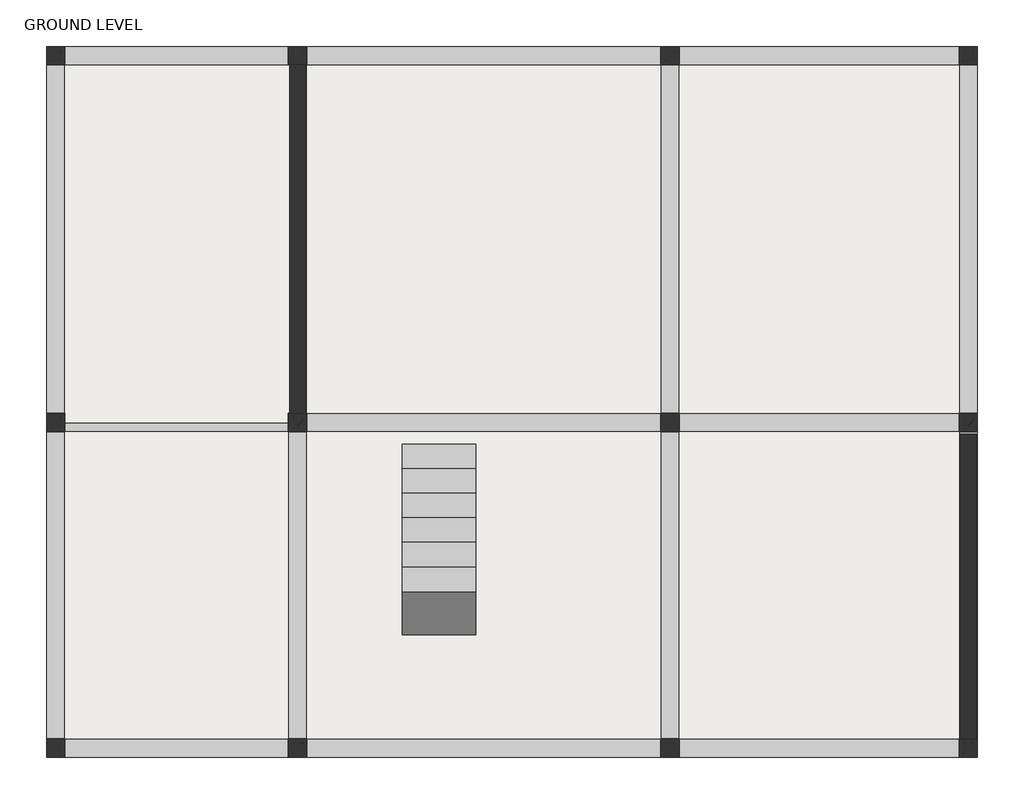
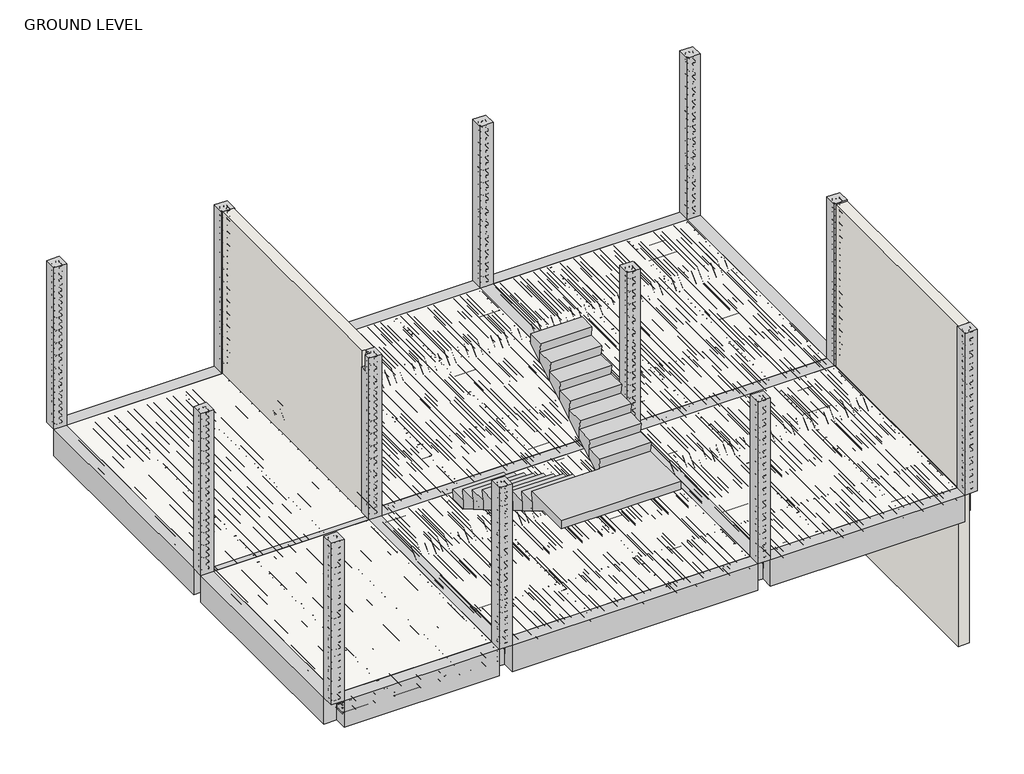
# One storey, part 1 of 8: 17 beams, 12 columns, 6 slabs, 2 walls, 1 stair flight.
"""IFC4 building model written with IfcOpenShell, lengths in millimetres."""

from ifc_helpers import new_model, si_unit, frame, origin, origin_with_axes, place, context, project, spatial, polyline, outline, extrude, faceted_brep, element, save

model = new_model("IFC4")

# Units and contexts
model_context = context("Model", 3, world=origin())
ifc_project = project(units=[si_unit("LENGTHUNIT", "METRE", prefix="MILLI")], contexts=[model_context])

# Site, building, storey
site = spatial("IfcSite", under=ifc_project)
building = spatial("IfcBuilding", under=site)
storey = spatial("IfcBuildingStorey", under=building, Name="GROUND LEVEL", Elevation=0.0)

# Beams
placement = place(None, origin())
element("IfcBeam", 1, ObjectType="M_Concrete-Rectangular Beam : BEAM 500MM X 500MM", at=placement, inside=storey, context=model_context, shape_type="Brep", body=[
    faceted_brep([(-12040.8556799, 4198.3016651, 0.0), (-12040.8556799, 4426.9016651, 0.0), (-14809.4556799, 4426.9016651, 0.0), (-14809.4556799, 4198.3016651, 0.0), (-12040.8556799, 4198.3016651, -500.0), (-14809.4556799, 4198.3016651, -300.0), (-14809.4556799, 4198.3016651, -500.0), (-12040.8556799, 4426.9016651, -500.0), (-14809.4556799, 4426.9016651, -500.0)], [[[0, 1, 2, 3]], [[4, 0, 3, 5, 6]], [[7, 4, 6, 8]], [[1, 7, 8, 2]], [[2, 8, 6, 5, 3]], [[1, 0, 4, 7]]]),
])
element("IfcBeam", 2, ObjectType="M_Concrete-Rectangular Beam : BEAM 500MM X 500MM", at=placement, inside=storey, context=model_context, shape_type="Brep", body=[
    faceted_brep([(-7428.7673382, 4198.3016651, 0.0), (-7428.7673382, 4426.9016651, 0.0), (-11812.2556799, 4426.9016651, 0.0), (-11812.2556799, 4198.3016651, 0.0), (-7428.7673382, 4198.3016651, -500.0), (-7428.7673382, 4198.3016651, -300.0), (-11812.2556799, 4198.3016651, -300.0), (-11812.2556799, 4198.3016651, -500.0), (-7428.7673382, 4426.9016651, -500.0), (-11812.2556799, 4426.9016651, -500.0)], [[[0, 1, 2, 3]], [[4, 5, 0, 3, 6, 7]], [[8, 4, 7, 9]], [[1, 8, 9, 2]], [[2, 9, 7, 6, 3]], [[1, 0, 5, 4, 8]]]),
])
element("IfcBeam", 3, ObjectType="M_Concrete-Rectangular Beam : BEAM 500MM X 500MM", at=placement, inside=storey, context=model_context, shape_type="Brep", body=[
    faceted_brep([(-3735.0556799, 4198.3016651, 0.0), (-3735.0556799, 4426.9016651, 0.0), (-7200.1673382, 4426.9016651, 0.0), (-7200.1673382, 4198.3016651, 0.0), (-3735.0556799, 4198.3016651, -500.0), (-3735.0556799, 4198.3016651, -300.0), (-7200.1673382, 4198.3016651, -300.0), (-7200.1673382, 4198.3016651, -500.0), (-3735.0556799, 4426.9016651, -500.0), (-7200.1673382, 4426.9016651, -500.0)], [[[0, 1, 2, 3]], [[4, 5, 0, 3, 6, 7]], [[8, 4, 7, 9]], [[1, 8, 9, 2]], [[2, 9, 7, 6, 3]], [[1, 0, 5, 4, 8]]]),
])
element("IfcBeam", 4, ObjectType="M_Concrete-Rectangular Beam : BEAM 500MM X 500MM", at=placement, inside=storey, context=model_context, shape_type="Brep", body=[
    faceted_brep([(-15038.0556799, -118.4025279, 0.0), (-14809.4556799, -118.4025279, 0.0), (-14809.4556799, 4198.3016651, 0.0), (-15038.0556799, 4198.3016651, 0.0), (-15038.0556799, -118.4025279, -500.0), (-15038.0556799, 4198.3016651, -500.0), (-14809.4556799, -118.4025279, -500.0), (-14809.4556799, 4198.3016651, -500.0), (-14809.4556799, 4198.3016651, -300.0)], [[[0, 1, 2, 3]], [[4, 0, 3, 5]], [[6, 4, 5, 7]], [[1, 6, 7, 8, 2]], [[2, 8, 7, 5, 3]], [[1, 0, 4, 6]]]),
])
element("IfcBeam", 5, ObjectType="M_Concrete-Rectangular Beam : BEAM 500MM X 500MM", at=placement, inside=storey, context=model_context, shape_type="Brep", body=[
    faceted_brep([(-14809.4556799, -347.0025279, 0.0), (-15038.0556799, -347.0025279, 0.0), (-15038.0556799, -4145.5983349, 0.0), (-14809.4556799, -4145.5983349, 0.0), (-15038.0556799, -347.0025279, -500.0), (-15038.0556799, -4145.5983349, -500.0), (-14809.4556799, -347.0025279, -500.0), (-14809.4556799, -4145.5983349, -500.0), (-14809.4556799, -347.0025279, -300.0), (-14809.4556799, -4145.5983349, -300.0)], [[[0, 1, 2, 3]], [[1, 4, 5, 2]], [[4, 6, 7, 5]], [[6, 8, 0, 3, 9, 7]], [[0, 8, 6, 4, 1]], [[3, 2, 5, 7, 9]]]),
])
element("IfcBeam", 6, ObjectType="M_Concrete-Rectangular Beam : BEAM 500MM X 500MM", at=placement, inside=storey, context=model_context, shape_type="Brep", body=[
    faceted_brep([(-12040.8556799, -4374.1983349, 0.0), (-12040.8556799, -4145.5983349, 0.0), (-14809.4556799, -4145.5983349, 0.0), (-14809.4556799, -4374.1983349, 0.0), (-12040.8556799, -4374.1983349, -500.0), (-14809.4556799, -4374.1983349, -500.0), (-12040.8556799, -4145.5983349, -500.0), (-14809.4556799, -4145.5983349, -500.0), (-12040.8556799, -4145.5983349, -300.0), (-14809.4556799, -4145.5983349, -300.0)], [[[0, 1, 2, 3]], [[4, 0, 3, 5]], [[6, 4, 5, 7]], [[1, 8, 6, 7, 9, 2]], [[2, 9, 7, 5, 3]], [[1, 0, 4, 6, 8]]]),
])
element("IfcBeam", 7, ObjectType="M_Concrete-Rectangular Beam : BEAM 500MM X 500MM", at=placement, inside=storey, context=model_context, shape_type="Brep", body=[
    faceted_brep([(-11812.2556799, -4145.5983349, 0.0), (-11812.2556799, -4374.1983349, 0.0), (-7428.7673382, -4374.1983349, 0.0), (-7428.7673382, -4145.5983349, 0.0), (-11812.2556799, -4374.1983349, -500.0), (-7428.7673382, -4374.1983349, -500.0), (-11812.2556799, -4145.5983349, -500.0), (-7428.7673382, -4145.5983349, -500.0), (-11812.2556799, -4145.5983349, -300.0), (-7428.7673382, -4145.5983349, -300.0)], [[[0, 1, 2, 3]], [[1, 4, 5, 2]], [[4, 6, 7, 5]], [[6, 8, 0, 3, 9, 7]], [[0, 8, 6, 4, 1]], [[3, 2, 5, 7, 9]]]),
])
element("IfcBeam", 8, ObjectType="M_Concrete-Rectangular Beam : BEAM 500MM X 500MM", at=placement, inside=storey, context=model_context, shape_type="Brep", body=[
    faceted_brep([(-7200.1673382, -4145.5983349, 0.0), (-7200.1673382, -4374.1983349, 0.0), (-3735.0556799, -4374.1983349, 0.0), (-3735.0556799, -4145.5983349, 0.0), (-7200.1673382, -4374.1983349, -500.0), (-3735.0556799, -4374.1983349, -500.0), (-7200.1673382, -4145.5983349, -500.0), (-3735.0556799, -4145.5983349, -500.0), (-7200.1673382, -4145.5983349, -300.0), (-3735.0556799, -4145.5983349, -300.0)], [[[0, 1, 2, 3]], [[1, 4, 5, 2]], [[4, 6, 7, 5]], [[6, 8, 0, 3, 9, 7]], [[0, 8, 6, 4, 1]], [[3, 2, 5, 7, 9]]]),
])
element("IfcBeam", 9, ObjectType="M_Concrete-Rectangular Beam : BEAM 500MM X 500MM", at=placement, inside=storey, context=model_context, shape_type="Brep", body=[
    faceted_brep([(-3735.0556799, -4145.5983349, 0.0), (-3506.4556799, -4145.5983349, 0.0), (-3506.4556799, -347.0025279, 0.0), (-3735.0556799, -347.0025279, 0.0), (-3506.4556799, -4145.5983349, -500.0), (-3506.4556799, -347.0025279, -500.0), (-3735.0556799, -4145.5983349, -500.0), (-3735.0556799, -347.0025279, -500.0), (-3735.0556799, -4145.5983349, -300.0), (-3735.0556799, -347.0025279, -300.0)], [[[0, 1, 2, 3]], [[1, 4, 5, 2]], [[4, 6, 7, 5]], [[6, 8, 0, 3, 9, 7]], [[0, 8, 6, 4, 1]], [[3, 2, 5, 7, 9]]]),
])
element("IfcBeam", 10, ObjectType="M_Concrete-Rectangular Beam : BEAM 500MM X 500MM", at=placement, inside=storey, context=model_context, shape_type="Brep", body=[
    faceted_brep([(-3506.4556799, 4198.3016651, 0.0), (-3735.0556799, 4198.3016651, 0.0), (-3735.0556799, -118.4025279, 0.0), (-3506.4556799, -118.4025279, 0.0), (-3506.4556799, 4198.3016651, -500.0), (-3506.4556799, -118.4025279, -500.0), (-3735.0556799, 4198.3016651, -500.0), (-3735.0556799, -118.4025279, -500.0), (-3735.0556799, 4198.3016651, -300.0), (-3735.0556799, -118.4025279, -300.0)], [[[0, 1, 2, 3]], [[4, 0, 3, 5]], [[6, 4, 5, 7]], [[1, 8, 6, 7, 9, 2]], [[1, 0, 4, 6, 8]], [[3, 2, 9, 7, 5]]]),
])
element("IfcBeam", 11, ObjectType="M_Concrete-Rectangular Beam : BEAM 500MM X 500MM", at=placement, inside=storey, context=model_context, shape_type="Brep", body=[
    faceted_brep([(-14809.4556799, -347.0025279, 0.0), (-12040.8556799, -347.0025279, 0.0), (-12040.8556799, -232.7025279, 0.0), (-14809.4556799, -232.7025279, 0.0), (-14809.4556799, -347.0025279, -300.0), (-14809.4556799, -347.0025279, -500.0), (-12040.8556799, -347.0025279, -500.0), (-12040.8556799, -347.0025279, -300.0), (-14809.4556799, -118.4025279, -500.0), (-12040.8556799, -118.4025279, -500.0), (-14809.4556799, -118.4025279, -300.0), (-12040.8556799, -118.4025279, -300.0), (-14809.4556799, -232.7025279, -300.0), (-12040.8556799, -232.7025279, -300.0)], [[[0, 1, 2, 3]], [[0, 4, 5, 6, 7, 1]], [[5, 8, 9, 6]], [[9, 8, 10, 11]], [[8, 5, 4, 0, 3, 12, 10]], [[1, 7, 6, 9, 11, 13, 2]], [[12, 13, 11, 10]], [[13, 12, 3, 2]]]),
])
element("IfcBeam", 12, ObjectType="M_Concrete-Rectangular Beam : BEAM 500MM X 500MM", at=placement, inside=storey, context=model_context, shape_type="Brep", body=[
    faceted_brep([(-11812.2556799, -118.4025279, 0.0), (-11812.2556799, -347.0025279, 0.0), (-7428.7673382, -347.0025279, 0.0), (-7428.7673382, -118.4025279, 0.0), (-11812.2556799, -347.0025279, -300.0), (-11812.2556799, -347.0025279, -500.0), (-7428.7673382, -347.0025279, -500.0), (-7428.7673382, -347.0025279, -300.0), (-11812.2556799, -118.4025279, -500.0), (-7428.7673382, -118.4025279, -500.0), (-11812.2556799, -118.4025279, -300.0), (-7428.7673382, -118.4025279, -300.0)], [[[0, 1, 2, 3]], [[1, 4, 5, 6, 7, 2]], [[5, 8, 9, 6]], [[8, 10, 0, 3, 11, 9]], [[0, 10, 8, 5, 4, 1]], [[3, 2, 7, 6, 9, 11]]]),
])
element("IfcBeam", 13, ObjectType="M_Concrete-Rectangular Beam : BEAM 500MM X 500MM", at=placement, inside=storey, context=model_context, shape_type="Brep", body=[
    faceted_brep([(-7200.1673382, -118.4025279, 0.0), (-7200.1673382, -347.0025279, 0.0), (-3735.0556799, -347.0025279, 0.0), (-3735.0556799, -118.4025279, 0.0), (-7200.1673382, -347.0025279, -300.0), (-7200.1673382, -347.0025279, -500.0), (-3735.0556799, -347.0025279, -500.0), (-3735.0556799, -347.0025279, -300.0), (-7200.1673382, -118.4025279, -500.0), (-3735.0556799, -118.4025279, -500.0), (-7200.1673382, -118.4025279, -300.0), (-3735.0556799, -118.4025279, -300.0)], [[[0, 1, 2, 3]], [[1, 4, 5, 6, 7, 2]], [[5, 8, 9, 6]], [[8, 10, 0, 3, 11, 9]], [[1, 0, 10, 8, 5, 4]], [[3, 2, 7, 6, 9, 11]]]),
])
element("IfcBeam", 14, ObjectType="M_Concrete-Rectangular Beam : BEAM 500MM X 500MM", at=placement, inside=storey, context=model_context, shape_type="Brep", body=[
    faceted_brep([(-11812.2556799, -118.4025279, 0.0), (-11812.2556799, 4198.3016651, 0.0), (-11964.6556799, 4198.3016651, 0.0), (-11964.6556799, -118.4025279, 0.0), (-12040.8556799, 4198.3016651, -500.0), (-12040.8556799, -118.4025279, -500.0), (-12040.8556799, -118.4025279, -300.0), (-12040.8556799, 4198.3016651, -300.0), (-11812.2556799, 4198.3016651, -500.0), (-11812.2556799, -118.4025279, -500.0), (-11812.2556799, -118.4025279, -300.0), (-11812.2556799, 4198.3016651, -300.0), (-11964.6556799, 4198.3016651, -300.0), (-11964.6556799, -118.4025279, -300.0)], [[[0, 1, 2, 3]], [[4, 5, 6, 7]], [[5, 4, 8, 9]], [[1, 0, 10, 9, 8, 11]], [[1, 11, 8, 4, 7, 12, 2]], [[5, 9, 10, 0, 3, 13, 6]], [[13, 12, 7, 6]], [[12, 13, 3, 2]]]),
])
element("IfcBeam", 15, ObjectType="M_Concrete-Rectangular Beam : BEAM 500MM X 500MM", at=placement, inside=storey, context=model_context, shape_type="Brep", body=[
    faceted_brep([(-11812.2556799, -347.0025279, 0.0), (-12040.8556799, -347.0025279, 0.0), (-12040.8556799, -4145.5983349, 0.0), (-11812.2556799, -4145.5983349, 0.0), (-12040.8556799, -347.0025279, -300.0), (-12040.8556799, -347.0025279, -500.0), (-12040.8556799, -4145.5983349, -500.0), (-12040.8556799, -4145.5983349, -300.0), (-11812.2556799, -347.0025279, -500.0), (-11812.2556799, -4145.5983349, -500.0), (-11812.2556799, -347.0025279, -300.0), (-11812.2556799, -4145.5983349, -300.0)], [[[0, 1, 2, 3]], [[1, 4, 5, 6, 7, 2]], [[5, 8, 9, 6]], [[8, 10, 0, 3, 11, 9]], [[0, 10, 8, 5, 4, 1]], [[3, 2, 7, 6, 9, 11]]]),
])
element("IfcBeam", 16, ObjectType="M_Concrete-Rectangular Beam : BEAM 500MM X 500MM", at=placement, inside=storey, context=model_context, shape_type="Brep", body=[
    faceted_brep([(-7200.1673382, -347.0025279, 0.0), (-7428.7673382, -347.0025279, 0.0), (-7428.7673382, -4145.5983349, 0.0), (-7200.1673382, -4145.5983349, 0.0), (-7200.1673382, -347.0025279, -500.0), (-7200.1673382, -347.0025279, -300.0), (-7200.1673382, -4145.5983349, -300.0), (-7200.1673382, -4145.5983349, -500.0), (-7428.7673382, -347.0025279, -500.0), (-7428.7673382, -4145.5983349, -500.0), (-7428.7673382, -347.0025279, -300.0), (-7428.7673382, -4145.5983349, -300.0)], [[[0, 1, 2, 3]], [[4, 5, 0, 3, 6, 7]], [[8, 4, 7, 9]], [[1, 10, 8, 9, 11, 2]], [[1, 0, 5, 4, 8, 10]], [[2, 11, 9, 7, 6, 3]]]),
])
element("IfcBeam", 17, ObjectType="M_Concrete-Rectangular Beam : BEAM 500MM X 500MM", at=placement, inside=storey, context=model_context, shape_type="Brep", body=[
    faceted_brep([(-7200.1673382, 4198.3016651, 0.0), (-7428.7673382, 4198.3016651, 0.0), (-7428.7673382, -118.4025279, 0.0), (-7200.1673382, -118.4025279, 0.0), (-7200.1673382, 4198.3016651, -500.0), (-7200.1673382, 4198.3016651, -300.0), (-7200.1673382, -118.4025279, -300.0), (-7200.1673382, -118.4025279, -500.0), (-7428.7673382, 4198.3016651, -500.0), (-7428.7673382, -118.4025279, -500.0), (-7428.7673382, 4198.3016651, -300.0), (-7428.7673382, -118.4025279, -300.0)], [[[0, 1, 2, 3]], [[4, 5, 0, 3, 6, 7]], [[8, 4, 7, 9]], [[1, 10, 8, 9, 11, 2]], [[1, 0, 5, 4, 8, 10]], [[2, 11, 9, 7, 6, 3]]]),
])

# Columns
element("IfcColumn", 18, ObjectType="M_Concrete-Rectangular-Column : 9\" X 9\"", at=placement, inside=storey, context=model_context, shape_type="SweptSolid", body=[
    extrude(outline(polyline([(-14809.4556799, 4426.9016651), (-14809.4556799, 4198.3016651), (-15038.0556799, 4198.3016651), (-15038.0556799, 4426.9016651), (-14809.4556799, 4426.9016651)])), origin_with_axes(), (0.0, 0.0, 1.0), 3048.0),
])
element("IfcColumn", 19, ObjectType="M_Concrete-Rectangular-Column : 9\" X 9\"", at=placement, inside=storey, context=model_context, shape_type="Brep", body=[
    faceted_brep([(-11812.2556799, 4426.9016651, 0.0), (-11812.2556799, 4198.3016651, 0.0), (-12040.8556799, 4198.3016651, 0.0), (-12040.8556799, 4426.9016651, 0.0), (-11812.2556799, 4426.9016651, 3048.0), (-11812.2556799, 4198.3016651, 3048.0), (-11964.6556799, 4198.3016651, 3048.0), (-12040.8556799, 4198.3016651, 3048.0), (-12040.8556799, 4426.9016651, 3048.0)], [[[0, 1, 2, 3]], [[4, 5, 1, 0]], [[5, 6, 7, 2, 1]], [[7, 8, 3, 2]], [[8, 4, 0, 3]], [[4, 8, 7, 6, 5]]]),
])
element("IfcColumn", 20, ObjectType="M_Concrete-Rectangular-Column : 9\" X 9\"", at=placement, inside=storey, context=model_context, shape_type="SweptSolid", body=[
    extrude(outline(polyline([(-7200.1673382, 4426.9016651), (-7200.1673382, 4198.3016651), (-7428.7673382, 4198.3016651), (-7428.7673382, 4426.9016651), (-7200.1673382, 4426.9016651)])), origin_with_axes(), (0.0, 0.0, 1.0), 3048.0),
])
element("IfcColumn", 21, ObjectType="M_Concrete-Rectangular-Column : 9\" X 9\"", at=placement, inside=storey, context=model_context, shape_type="SweptSolid", body=[
    extrude(outline(polyline([(-3506.4556799, 4426.9016651), (-3506.4556799, 4198.3016651), (-3735.0556799, 4198.3016651), (-3735.0556799, 4426.9016651), (-3506.4556799, 4426.9016651)])), origin_with_axes(), (0.0, 0.0, 1.0), 3048.0),
])
element("IfcColumn", 22, ObjectType="M_Concrete-Rectangular-Column : 9\" X 9\"", at=placement, inside=storey, context=model_context, shape_type="SweptSolid", body=[
    extrude(outline(polyline([(-3506.4556799, -118.4025279), (-3506.4556799, -347.0025279), (-3735.0556799, -347.0025279), (-3735.0556799, -118.4025279), (-3506.4556799, -118.4025279)])), origin_with_axes(), (0.0, 0.0, 1.0), 3048.0),
])
element("IfcColumn", 23, ObjectType="M_Concrete-Rectangular-Column : 9\" X 9\"", at=placement, inside=storey, context=model_context, shape_type="SweptSolid", body=[
    extrude(outline(polyline([(-7200.1673382, -118.4025279), (-7200.1673382, -347.0025279), (-7428.7673382, -347.0025279), (-7428.7673382, -118.4025279), (-7200.1673382, -118.4025279)])), origin_with_axes(), (0.0, 0.0, 1.0), 3048.0),
])
element("IfcColumn", 24, ObjectType="M_Concrete-Rectangular-Column : 9\" X 9\"", at=placement, inside=storey, context=model_context, shape_type="Brep", body=[
    faceted_brep([(-11812.2556799, -118.4025279, 0.0), (-11812.2556799, -347.0025279, 0.0), (-12040.8556799, -347.0025279, 0.0), (-12040.8556799, -118.4025279, 0.0), (-11812.2556799, -118.4025279, 3048.0), (-11812.2556799, -347.0025279, 3048.0), (-12040.8556799, -347.0025279, 3048.0), (-12040.8556799, -232.7025279, 3048.0), (-12040.8556799, -232.7025279, 2748.0), (-12040.8556799, -118.4025279, 2748.0), (-11964.6556799, -118.4025279, 2748.0), (-11964.6556799, -118.4025279, 3048.0), (-11964.6556799, -232.7025279, 3048.0), (-11964.6556799, -232.7025279, 2748.0)], [[[0, 1, 2, 3]], [[1, 0, 4, 5]], [[2, 1, 5, 6]], [[3, 2, 6, 7, 8, 9]], [[0, 3, 9, 10, 11, 4]], [[5, 4, 11, 12, 7, 6]], [[8, 13, 10, 9]], [[13, 12, 11, 10]], [[12, 13, 8, 7]]]),
])
element("IfcColumn", 25, ObjectType="M_Concrete-Rectangular-Column : 9\" X 9\"", at=placement, inside=storey, context=model_context, shape_type="Brep", body=[
    faceted_brep([(-14809.4556799, -118.4025279, 0.0), (-14809.4556799, -347.0025279, 0.0), (-15038.0556799, -347.0025279, 0.0), (-15038.0556799, -118.4025279, 0.0), (-14809.4556799, -118.4025279, 3048.0), (-14809.4556799, -232.7025279, 3048.0), (-14809.4556799, -347.0025279, 3048.0), (-15038.0556799, -347.0025279, 3048.0), (-15038.0556799, -118.4025279, 3048.0)], [[[0, 1, 2, 3]], [[4, 5, 6, 1, 0]], [[6, 7, 2, 1]], [[7, 8, 3, 2]], [[8, 4, 0, 3]], [[4, 8, 7, 6, 5]]]),
])
element("IfcColumn", 26, ObjectType="M_Concrete-Rectangular-Column : 9\" X 9\"", at=placement, inside=storey, context=model_context, shape_type="SweptSolid", body=[
    extrude(outline(polyline([(-14809.4556799, -4145.5983349), (-14809.4556799, -4374.1983349), (-15038.0556799, -4374.1983349), (-15038.0556799, -4145.5983349), (-14809.4556799, -4145.5983349)])), origin_with_axes(), (0.0, 0.0, 1.0), 3048.0),
])
element("IfcColumn", 27, ObjectType="M_Concrete-Rectangular-Column : 9\" X 9\"", at=placement, inside=storey, context=model_context, shape_type="SweptSolid", body=[
    extrude(outline(polyline([(-11812.2556799, -4145.5983349), (-11812.2556799, -4374.1983349), (-12040.8556799, -4374.1983349), (-12040.8556799, -4145.5983349), (-11812.2556799, -4145.5983349)])), origin_with_axes(), (0.0, 0.0, 1.0), 3048.0),
])
element("IfcColumn", 28, ObjectType="M_Concrete-Rectangular-Column : 9\" X 9\"", at=placement, inside=storey, context=model_context, shape_type="SweptSolid", body=[
    extrude(outline(polyline([(-7200.1673382, -4145.5983349), (-7200.1673382, -4374.1983349), (-7428.7673382, -4374.1983349), (-7428.7673382, -4145.5983349), (-7200.1673382, -4145.5983349)])), origin_with_axes(), (0.0, 0.0, 1.0), 3048.0),
])
element("IfcColumn", 29, ObjectType="M_Concrete-Rectangular-Column : 9\" X 9\"", at=placement, inside=storey, context=model_context, shape_type="SweptSolid", body=[
    extrude(outline(polyline([(-3506.4556799, -4145.5983349), (-3506.4556799, -4374.1983349), (-3735.0556799, -4374.1983349), (-3735.0556799, -4145.5983349), (-3506.4556799, -4145.5983349)])), origin_with_axes(), (0.0, 0.0, 1.0), 3048.0),
])

# Slabs
element("IfcSlab", 30, ObjectType="Generic 300mm", at=placement, inside=storey, context=model_context, shape_type="Brep", body=[
    faceted_brep([(-11964.6556799, 4198.3016651, -300.0), (-11964.6556799, -118.4025279, -300.0), (-11964.6556799, -232.7025279, -300.0), (-12040.8556799, -232.7025279, -300.0), (-14809.4556799, -232.7025279, -300.0), (-14809.4556799, -118.4025279, -300.0), (-14809.4556799, 4198.3016651, -300.0), (-12040.8556799, 4198.3016651, -300.0), (-11964.6556799, 4198.3016651, 0.0), (-12040.8556799, 4198.3016651, 0.0), (-14809.4556799, 4198.3016651, 0.0), (-14809.4556799, -118.4025279, 0.0), (-14809.4556799, -232.7025279, 0.0), (-12040.8556799, -232.7025279, 0.0), (-11964.6556799, -232.7025279, 0.0), (-11964.6556799, -118.4025279, 0.0)], [[[0, 1, 2, 3, 4, 5, 6, 7]], [[8, 9, 10, 11, 12, 13, 14, 15]], [[2, 1, 0, 8, 15, 14]], [[4, 3, 2, 14, 13, 12]], [[6, 5, 4, 12, 11, 10]], [[0, 7, 6, 10, 9, 8]]]),
])
element("IfcSlab", 31, ObjectType="Generic 300mm", at=placement, inside=storey, context=model_context, shape_type="SweptSolid", body=[
    extrude(outline(polyline([(-7428.7673382, 4198.3016651), (-7428.7673382, -118.4025279), (-11812.2556799, -118.4025279), (-11812.2556799, 4198.3016651), (-7428.7673382, 4198.3016651)])), frame((0.0, 0.0, -300.0), z_axis=(0.0, 0.0, 1.0), x_axis=(1.0, 0.0, 0.0)), (0.0, 0.0, 1.0), 300.0),
])
element("IfcSlab", 32, ObjectType="Generic 300mm", at=placement, inside=storey, context=model_context, shape_type="SweptSolid", body=[
    extrude(outline(polyline([(-3735.0556799, 4198.3016651), (-3735.0556799, -118.4025279), (-7200.1673382, -118.4025279), (-7200.1673382, 4198.3016651), (-3735.0556799, 4198.3016651)])), frame((0.0, 0.0, -300.0), z_axis=(0.0, 0.0, 1.0), x_axis=(1.0, 0.0, 0.0)), (0.0, 0.0, 1.0), 300.0),
])
element("IfcSlab", 33, ObjectType="Generic 300mm", at=placement, inside=storey, context=model_context, shape_type="SweptSolid", body=[
    extrude(outline(polyline([(-12040.8556799, -347.0025279), (-12040.8556799, -4145.5983349), (-14809.4556799, -4145.5983349), (-14809.4556799, -347.0025279), (-12040.8556799, -347.0025279)])), frame((0.0, 0.0, -300.0), z_axis=(0.0, 0.0, 1.0), x_axis=(1.0, 0.0, 0.0)), (0.0, 0.0, 1.0), 300.0),
])
element("IfcSlab", 34, ObjectType="Generic 300mm", at=placement, inside=storey, context=model_context, shape_type="SweptSolid", body=[
    extrude(outline(polyline([(-7428.7673382, -347.0025279), (-7428.7673382, -4145.5983349), (-11812.2556799, -4145.5983349), (-11812.2556799, -347.0025279), (-7428.7673382, -347.0025279)])), frame((0.0, 0.0, -300.0), z_axis=(0.0, 0.0, 1.0), x_axis=(1.0, 0.0, 0.0)), (0.0, 0.0, 1.0), 300.0),
])
element("IfcSlab", 35, ObjectType="Generic 300mm", at=placement, inside=storey, context=model_context, shape_type="SweptSolid", body=[
    extrude(outline(polyline([(-3735.0556799, -347.0025279), (-3735.0556799, -4145.5983349), (-7200.1673382, -4145.5983349), (-7200.1673382, -347.0025279), (-3735.0556799, -347.0025279)])), frame((0.0, 0.0, -300.0), z_axis=(0.0, 0.0, 1.0), x_axis=(1.0, 0.0, 0.0)), (0.0, 0.0, 1.0), 300.0),
])

# Stair flight
element("IfcStairFlight", 36, ObjectType="25 mm Nosing", at=placement, inside=storey, context=model_context, shape_type="Brep", body=[
    faceted_brep([(-10633.5476583, -496.8755812, 179.2941176), (-9719.1476583, -496.8755812, 179.2941176), (-9719.1476583, -521.8755812, 0.0), (-10633.5476583, -521.8755812, 0.0), (-10633.5476583, -826.6755812, 179.2941176), (-9719.1476583, -826.6755812, 179.2941176), (-9719.1476583, -826.6755812, 5.2669154), (-9719.1476583, -817.7218251, 0.0), (-10633.5476583, -817.7218251, 0.0), (-10633.5476583, -826.6755812, 5.2669154), (-9719.1476583, -801.6755812, 358.5882353), (-10633.5476583, -801.6755812, 358.5882353), (-10633.5476583, -1131.4755812, 358.5882353), (-9719.1476583, -1131.4755812, 358.5882353), (-9719.1476583, -1131.4755812, 184.561033), (-10633.5476583, -1131.4755812, 184.561033), (-9719.1476583, -1106.4755812, 537.8823529), (-10633.5476583, -1106.4755812, 537.8823529), (-10633.5476583, -1436.2755812, 537.8823529), (-9719.1476583, -1436.2755812, 537.8823529), (-9719.1476583, -1436.2755812, 363.8551507), (-10633.5476583, -1436.2755812, 363.8551507), (-9719.1476583, -1411.2755812, 717.1764706), (-10633.5476583, -1411.2755812, 717.1764706), (-10633.5476583, -1741.0755812, 717.1764706), (-9719.1476583, -1741.0755812, 717.1764706), (-9719.1476583, -1741.0755812, 543.1492683), (-10633.5476583, -1741.0755812, 543.1492683), (-9719.1476583, -1716.0755812, 896.4705882), (-10633.5476583, -1716.0755812, 896.4705882), (-10633.5476583, -2045.8755812, 896.4705882), (-9719.1476583, -2045.8755812, 896.4705882), (-9719.1476583, -2045.8755812, 722.443386), (-10633.5476583, -2045.8755812, 722.443386), (-9719.1476583, -2020.8755812, 1075.7647059), (-10633.5476583, -2020.8755812, 1075.7647059), (-10633.5476583, -2350.6755812, 1075.7647059), (-9719.1476583, -2350.6755812, 1075.7647059), (-9719.1476583, -2350.6755812, 901.7375036), (-10633.5476583, -2350.6755812, 901.7375036), (-9719.1476583, -2325.6755812, 1255.0588235), (-10633.5476583, -2325.6755812, 1255.0588235), (-10633.5476583, -2655.4755812, 1255.0588235), (-9719.1476583, -2655.4755812, 1255.0588235), (-9719.1476583, -2655.4755812, 1081.0316213), (-10633.5476583, -2655.4755812, 1081.0316213), (-9719.1476583, -2960.2755812, 1434.3529412), (-9719.1476583, -2630.4755812, 1434.3529412), (-10633.5476583, -2630.4755812, 1434.3529412), (-10633.5476583, -2960.2755812, 1434.3529412), (-9719.1476583, -2956.1909355, 1463.6470588), (-9719.1476583, -3305.9218251, 1463.6470588), (-10633.5476583, -2960.2755812, 1260.3257389), (-9414.3476583, -2910.2755812, 1613.6470588), (-9414.3476583, -2935.2755812, 1613.6470588), (-9719.1476583, -2935.2755812, 1613.6470588), (-10633.5476583, -2935.2755812, 1613.6470588), (-10633.5476583, -3305.9218251, 1613.6470588), (-10633.5476583, -3849.6755812, 1613.6470588), (-8499.9476583, -3849.6755812, 1613.6470588), (-8499.9476583, -2910.2755812, 1613.6470588), (-9414.3476583, -2910.2755812, 1463.6470588), (-9414.3476583, -2935.2755812, 1463.6470588), (-9719.1476583, -2935.2755812, 1463.6470588), (-10633.5476583, -3305.9218251, 1463.6470588), (-10633.5476583, -3849.6755812, 1463.6470588), (-8499.9476583, -3849.6755812, 1463.6470588), (-8499.9476583, -2910.2755812, 1463.6470588), (-9414.3476583, -2935.2755812, 1792.9411765), (-8499.9476583, -2935.2755812, 1792.9411765), (-8499.9476583, -2869.4293374, 1792.9411765), (-8499.9476583, -2605.4755812, 1792.9411765), (-9414.3476583, -2605.4755812, 1792.9411765), (-9414.3476583, -2869.4293374, 1792.9411765), (-9414.3476583, -2605.4755812, 1618.9139742), (-9414.3476583, -2869.4293374, 1463.6470588), (-8499.9476583, -2869.4293374, 1463.6470588), (-8499.9476583, -2605.4755812, 1618.9139742), (-9414.3476583, -2630.4755812, 1972.2352941), (-8499.9476583, -2630.4755812, 1972.2352941), (-8499.9476583, -2300.6755812, 1972.2352941), (-9414.3476583, -2300.6755812, 1972.2352941), (-9414.3476583, -2300.6755812, 1798.2080919), (-8499.9476583, -2300.6755812, 1798.2080919), (-9414.3476583, -2325.6755812, 2151.5294118), (-8499.9476583, -2325.6755812, 2151.5294118), (-8499.9476583, -1995.8755812, 2151.5294118), (-9414.3476583, -1995.8755812, 2151.5294118), (-9414.3476583, -1995.8755812, 1977.5022095), (-8499.9476583, -1995.8755812, 1977.5022095), (-9414.3476583, -2020.8755812, 2330.8235294), (-8499.9476583, -2020.8755812, 2330.8235294), (-8499.9476583, -1691.0755812, 2330.8235294), (-9414.3476583, -1691.0755812, 2330.8235294), (-9414.3476583, -1691.0755812, 2156.7963271), (-8499.9476583, -1691.0755812, 2156.7963271), (-9414.3476583, -1716.0755812, 2510.1176471), (-8499.9476583, -1716.0755812, 2510.1176471), (-8499.9476583, -1386.2755812, 2510.1176471), (-9414.3476583, -1386.2755812, 2510.1176471), (-9414.3476583, -1386.2755812, 2336.0904448), (-8499.9476583, -1386.2755812, 2336.0904448), (-9414.3476583, -1411.2755812, 2689.4117647), (-8499.9476583, -1411.2755812, 2689.4117647), (-8499.9476583, -1081.4755812, 2689.4117647), (-9414.3476583, -1081.4755812, 2689.4117647), (-9414.3476583, -1081.4755812, 2515.3845624), (-8499.9476583, -1081.4755812, 2515.3845624), (-9414.3476583, -1106.4755812, 2868.7058824), (-8499.9476583, -1106.4755812, 2868.7058824), (-8499.9476583, -801.6755812, 2868.7058824), (-9414.3476583, -801.6755812, 2868.7058824), (-9414.3476583, -801.6755812, 2679.9727977), (-8499.9476583, -801.6755812, 2679.9727977)], [[[0, 1, 2, 3]], [[1, 0, 4, 5]], [[1, 5, 6, 7, 2]], [[4, 0, 3, 8, 9]], [[10, 11, 12, 13]], [[10, 13, 14, 6, 5]], [[12, 11, 4, 9, 15]], [[5, 4, 11, 10]], [[16, 17, 18, 19]], [[16, 19, 20, 14, 13]], [[18, 17, 12, 15, 21]], [[13, 12, 17, 16]], [[22, 23, 24, 25]], [[22, 25, 26, 20, 19]], [[24, 23, 18, 21, 27]], [[19, 18, 23, 22]], [[28, 29, 30, 31]], [[28, 31, 32, 26, 25]], [[30, 29, 24, 27, 33]], [[25, 24, 29, 28]], [[34, 35, 36, 37]], [[34, 37, 38, 32, 31]], [[36, 35, 30, 33, 39]], [[31, 30, 35, 34]], [[40, 41, 42, 43]], [[40, 43, 44, 38, 37]], [[42, 41, 36, 39, 45]], [[37, 36, 41, 40]], [[46, 47, 48, 49]], [[46, 50, 51, 44, 43, 47]], [[49, 48, 42, 45, 52]], [[43, 42, 48, 47]], [[53, 54, 55, 56, 57, 58, 59, 60]], [[54, 53, 61, 62]], [[55, 54, 62, 63]], [[50, 55, 63]], [[56, 49, 52, 64, 65, 58, 57]], [[59, 58, 65, 66]], [[60, 59, 66, 67]], [[46, 49, 56, 55, 50]], [[68, 69, 70, 71, 72, 73]], [[53, 68, 73, 72, 74, 75, 61]], [[69, 60, 67, 76, 77, 71, 70]], [[53, 60, 69, 68]], [[78, 79, 80, 81]], [[78, 81, 82, 74, 72]], [[80, 79, 71, 77, 83]], [[72, 71, 79, 78]], [[84, 85, 86, 87]], [[84, 87, 88, 82, 81]], [[86, 85, 80, 83, 89]], [[81, 80, 85, 84]], [[90, 91, 92, 93]], [[90, 93, 94, 88, 87]], [[92, 91, 86, 89, 95]], [[87, 86, 91, 90]], [[96, 97, 98, 99]], [[96, 99, 100, 94, 93]], [[98, 97, 92, 95, 101]], [[93, 92, 97, 96]], [[102, 103, 104, 105]], [[102, 105, 106, 100, 99]], [[104, 103, 98, 101, 107]], [[99, 98, 103, 102]], [[108, 109, 110, 111]], [[108, 111, 112, 106, 105]], [[110, 109, 104, 107, 113]], [[111, 110, 113, 112]], [[105, 104, 109, 108]], [[3, 2, 7, 8]], [[44, 51, 64, 52, 45, 39, 33, 27, 21, 15, 9, 8, 7, 6, 14, 20, 26, 32, 38]], [[64, 51, 50, 63, 62, 61, 75, 76, 67, 66, 65]], [[76, 75, 74, 82, 88, 94, 100, 106, 112, 113, 107, 101, 95, 89, 83, 77]]]),
])

# Walls
element("IfcWall", 37, ObjectType="Generic - 200mm", at=placement, inside=storey, context=model_context, shape_type="SweptSolid", body=[
    extrude(outline(polyline([(-3520.7556799, -373.6983349), (-3520.7556799, -4145.5983349), (-3720.7556799, -4145.5983349), (-3720.7556799, -373.6983349), (-3520.7556799, -373.6983349)])), frame((0.0, 0.0, -3000.0), z_axis=(0.0, 0.0, 1.0), x_axis=(1.0, 0.0, 0.0)), (0.0, 0.0, 1.0), 6048.0),
])
element("IfcWall", 38, ObjectType="Generic - 200mm", at=placement, inside=storey, context=model_context, shape_type="SweptSolid", body=[
    extrude(outline(polyline([(-12026.5556799, -118.4025279), (-12026.5556799, 4198.3016651), (-11826.5556799, 4198.3016651), (-11826.5556799, -118.4025279), (-12026.5556799, -118.4025279)])), frame((0.0, 0.0, -3000.0), z_axis=(0.0, 0.0, 1.0), x_axis=(1.0, 0.0, 0.0)), (0.0, 0.0, 1.0), 6048.0),
])

save(model, "model.ifc")

# Revit data of these elements
# Type "M_Concrete-Rectangular Beam : BEAM 500MM X 500MM"
#   Length [instance default] = 5' - 0"
#   b = 0' - 9"
#   h = 1' - 7.68504"
#   Structural Material [instance default] = Concrete, Cast-in-Place gray
#   Assembly Code = ""
# Type "M_Concrete-Rectangular-Column : 9\" X 9\""
#   b = 0' - 9"
#   h = 0' - 9"
#   Structural Material [instance default] = Concrete, Cast-in-Place gray
# Type "Generic 300mm"
#   Function = 0
#   Layers, outside or top first: 0' - 11.81102" no material (function 1)
# Type "Generic - 200mm"
#   Layers, outside or top first: 0' - 7.87402" no material (function 1)
# Elements 1, 2, 3, 4, 5, 6, 7, 8, 9, 10, 11, 12, 13, 14, 15, 16, 17 (IfcBeam, "M_Concrete-Rectangular Beam : BEAM 500MM X 500MM")
#   Structural Material = Concrete, Cast-in-Place gray
#   Phase Created = New Construction
#   Materials on its faces: "Concrete, Cast-in-Place gray"
# Elements 18, 19, 20, 21, 22, 23, 24, 25, 26, 27, 28, 29 (IfcColumn, "M_Concrete-Rectangular-Column : 9\" X 9\"")
#   Structural Material = Concrete, Cast-in-Place gray
#   Phase Created = New Construction
#   Materials on its faces: "Concrete, Cast-in-Place gray"
# Elements 30, 31, 32, 33, 34, 35 (IfcSlab, "Generic 300mm")
#   Height Offset From Level = 0' - 0"
#   built-in parameter 1001954 = 1
#   Phase Created = New Construction
#   Materials on its faces: "Default Floor"
# Element 36 (IfcStairFlight, "25 mm Nosing")
#   Phase Created = New Construction
#   Materials on its faces: "Concrete, Cast In Situ"
# Elements 37, 38 (IfcWall, "Generic - 200mm")
#   built-in parameter 1001111 = -9' - 10.11024"
#   Top Offset = 0' - 0"
#   Base Offset = -9' - 10.11024"
#   wall height = 19' - 10.11024"
#   Phase Created = New Construction
#   Base Constraint = GROUND LEVEL
#   Top Constraint = FIRST FLR
#   Materials on its faces: "Default Wall"
# Materials
#   "Concrete, Cast-in-Place gray": class "Concrete", colour RGB 192 192 192, transparency 0, Description = "Cast-in-place concrete", Cost = 0
#   "Default Floor": colour RGB 127 127 127, transparency 0, Cost = 0
#   "Concrete, Cast In Situ": class "Concrete", colour RGB 192 192 192, transparency 0, Description = "physical material", Cost = 0
#   "Default Wall": colour RGB 128 128 128, transparency 0, Cost = 0
